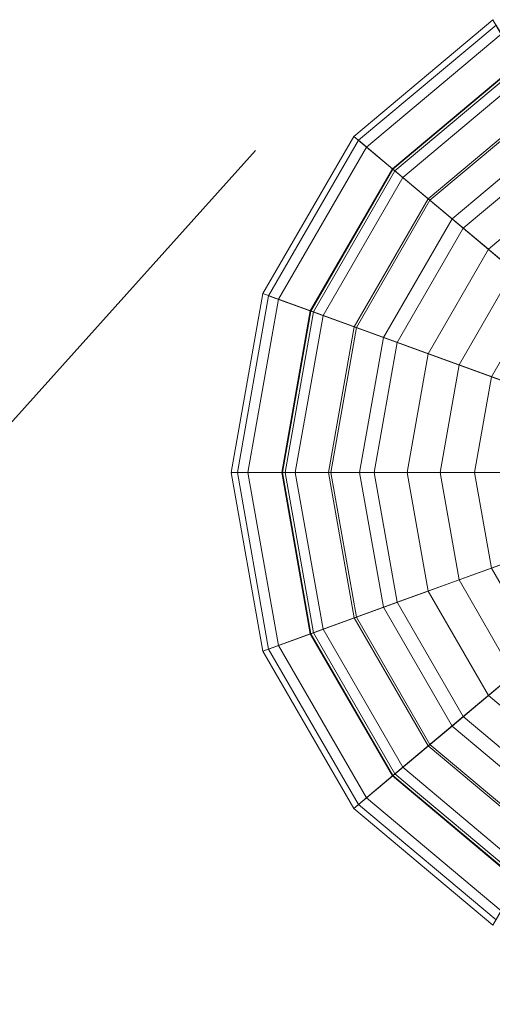
# Model space of a CAD drawing. Units: inches. Extents: x 375 to 1122, y 27 to 1069.
# Tile 57 of 155: x 731.16 to 732.383, y 305.711 to 308.262. Entities that reach past the tile are written whole.
import ezdxf

# ---------------------------------------------------------------- set-up
doc = ezdxf.new("R2010")
doc.units = ezdxf.units.IN
doc.layers.add('Furniture', color=30, linetype='Continuous', lineweight=18)

# ---------------------------------------------------------------- blocks, each defined once
blk = doc.blocks.new('A$C403C54AD')
blk.add_line((0.959313, 1.170619, -0.000599), (1.358468, 0.812559, -0.000599))
for points in [[(0.950832, 1.185986, -0.04658), (0.980157, 1.202917, -0.043501), (0.980157, 1.202917, -0.043501), (0.958391, 1.176977, -0.04658)], [(0.958391, 1.176977, -0.04658), (0.980157, 1.202917, -0.043501), (0.980157, 1.202917, -0.043501), (0.968576, 1.171097, -0.04658)], [(0.968576, 1.171097, -0.04658), (0.980157, 1.202917, -0.043501), (0.980157, 1.202917, -0.043501), (0.980157, 1.169055, -0.04658)], [(1.001923, 1.176977, -0.04658), (0.980157, 1.202917, -0.043501), (0.980157, 1.202917, -0.043501), (1.009483, 1.185986, -0.04658)], [(0.991739, 1.171097, -0.04658), (0.980157, 1.202917, -0.043501), (0.980157, 1.202917, -0.043501), (1.001923, 1.176977, -0.04658)], [(0.980157, 1.169055, -0.04658), (0.980157, 1.202917, -0.043501), (0.980157, 1.202917, -0.043501), (0.991739, 1.171097, -0.04658)], [(0.974434, 1.196096, 0.042248), (0.968505, 1.189031, 0.048884), (0.973957, 1.185883, 0.048884), (0.977112, 1.19455, 0.042248)], [(0.983203, 1.19455, 0.042248), (0.986357, 1.185883, 0.048884), (0.991809, 1.189031, 0.048884), (0.985881, 1.196096, 0.042248)], [(0.967847, 1.19581, -0.040074), (0.95366, 1.187619, -0.043349), (0.96049, 1.179479, -0.043349), (0.971021, 1.192029, -0.040074)], [(0.989294, 1.192029, -0.040074), (0.999824, 1.179479, -0.043349), (1.006655, 1.187619, -0.043349), (0.992467, 1.19581, -0.040074)], [(0.967072, 1.187323, 0.046697), (0.973653, 1.195166, 0.03933), (0.976696, 1.193409, 0.03933), (0.973195, 1.183788, 0.046697)], [(0.98712, 1.183788, 0.046697), (0.983618, 1.193409, 0.03933), (0.986661, 1.195166, 0.03933), (0.993243, 1.187323, 0.046697)], [(0.977112, 1.19455, 0.042248), (0.973957, 1.185883, 0.048884), (0.980157, 1.18479, 0.048884), (0.980157, 1.194013, 0.042248)], [(0.980157, 1.194013, 0.042248), (0.980157, 1.18479, 0.048884), (0.986357, 1.185883, 0.048884), (0.983203, 1.19455, 0.042248)], [(0.964459, 1.193854, 0.048884), (0.958842, 1.190611, 0.058276), (0.964336, 1.184063, 0.058276), (0.968505, 1.189031, 0.048884)], [(0.973195, 1.183788, 0.046697), (0.976696, 1.193409, 0.03933), (0.980157, 1.192799, 0.03933), (0.980157, 1.18256, 0.046697)], [(0.980157, 1.18256, 0.046697), (0.980157, 1.192799, 0.03933), (0.983618, 1.193409, 0.03933), (0.98712, 1.183788, 0.046697)], [(0.991809, 1.189031, 0.048884), (0.995978, 1.184063, 0.058276), (1.001473, 1.190611, 0.058276), (0.995856, 1.193854, 0.048884)], [(0.956408, 1.189206, 0.056929), (0.962527, 1.192739, 0.046697), (0.967072, 1.187323, 0.046697), (0.96253, 1.18191, 0.056929)], [(0.997785, 1.18191, 0.056929), (0.993243, 1.187323, 0.046697), (0.997787, 1.192739, 0.046697), (1.003907, 1.189206, 0.056929)], [(0.956282, 1.189133, 0.115599), (0.960688, 1.191677, 0.12581), (0.965707, 1.185696, 0.12581), (0.962436, 1.181798, 0.115599)], [(0.960688, 1.191677, 0.12581), (0.958022, 1.190138, 0.12581), (0.963728, 1.183338, 0.12581), (0.965707, 1.185696, 0.12581)], [(0.971021, 1.192029, -0.040074), (0.96049, 1.179479, -0.043349), (0.969693, 1.174166, -0.043349), (0.975296, 1.18956, -0.040074)], [(0.985019, 1.18956, -0.040074), (0.990622, 1.174166, -0.043349), (0.999824, 1.179479, -0.043349), (0.989294, 1.192029, -0.040074)], [(0.994608, 1.185696, 0.12581), (0.996587, 1.183338, 0.12581), (1.002293, 1.190138, 0.12581), (0.999627, 1.191677, 0.12581)], [(0.997878, 1.181798, 0.115599), (0.994608, 1.185696, 0.12581), (0.999627, 1.191677, 0.12581), (1.004033, 1.189133, 0.115599)], [(0.958842, 1.190611, 0.058276), (0.954418, 1.188057, 0.075423), (0.961053, 1.18015, 0.075423), (0.964336, 1.184063, 0.058276)], [(0.995978, 1.184063, 0.058276), (0.999261, 1.18015, 0.075423), (1.005896, 1.188057, 0.075423), (1.001473, 1.190611, 0.058276)], [(0.958022, 1.190138, 0.12581), (0.953695, 1.187639, 0.116404), (0.960516, 1.17951, 0.116404), (0.963728, 1.183338, 0.12581)], [(0.975296, 1.18956, -0.040074), (0.969693, 1.174166, -0.043349), (0.980157, 1.172321, -0.043349), (0.980157, 1.188703, -0.040074)], [(0.980157, 1.188703, -0.040074), (0.980157, 1.172321, -0.043349), (0.990622, 1.174166, -0.043349), (0.985019, 1.18956, -0.040074)], [(0.996587, 1.183338, 0.12581), (0.999798, 1.17951, 0.116404), (1.00662, 1.187639, 0.116404), (1.002293, 1.190138, 0.12581)], [(0.951762, 1.186523, 0.074938), (0.956408, 1.189206, 0.056929), (0.96253, 1.18191, 0.056929), (0.959081, 1.1778, 0.074938)], [(0.953848, 1.187728, 0.102963), (0.956282, 1.189133, 0.115599), (0.962436, 1.181798, 0.115599), (0.96063, 1.179646, 0.102963)], [(0.968505, 1.189031, 0.048884), (0.964336, 1.184063, 0.058276), (0.971739, 1.179789, 0.058276), (0.973957, 1.185883, 0.048884)], [(0.986357, 1.185883, 0.048884), (0.988575, 1.179789, 0.058276), (0.995978, 1.184063, 0.058276), (0.991809, 1.189031, 0.048884)], [(1.001233, 1.1778, 0.074938), (0.997785, 1.18191, 0.056929), (1.003907, 1.189206, 0.056929), (1.008553, 1.186523, 0.074938)], [(0.999684, 1.179646, 0.102963), (0.997878, 1.181798, 0.115599), (1.004033, 1.189133, 0.115599), (1.006466, 1.187728, 0.102963)], [(0.953695, 1.187639, 0.116404), (0.951177, 1.186186, 0.10318), (0.958647, 1.177283, 0.10318), (0.960516, 1.17951, 0.116404)], [(0.954418, 1.188057, 0.075423), (0.953848, 1.187728, 0.102963), (0.96063, 1.179646, 0.102963), (0.961053, 1.18015, 0.075423)], [(0.999261, 1.18015, 0.075423), (0.999684, 1.179646, 0.102963), (1.006466, 1.187728, 0.102963), (1.005896, 1.188057, 0.075423)], [(0.999798, 1.17951, 0.116404), (1.001667, 1.177283, 0.10318), (1.009137, 1.186186, 0.10318), (1.00662, 1.187639, 0.116404)], [(0.95366, 1.187619, -0.043349), (0.950832, 1.185986, -0.04658), (0.958391, 1.176977, -0.04658), (0.96049, 1.179479, -0.043349)], [(0.96253, 1.18191, 0.056929), (0.967072, 1.187323, 0.046697), (0.973195, 1.183788, 0.046697), (0.970778, 1.177147, 0.056929)], [(0.989537, 1.177147, 0.056929), (0.98712, 1.183788, 0.046697), (0.993243, 1.187323, 0.046697), (0.997785, 1.18191, 0.056929)], [(0.999824, 1.179479, -0.043349), (1.001923, 1.176977, -0.04658), (1.009483, 1.185986, -0.04658), (1.006655, 1.187619, -0.043349)], [(0.951177, 1.186186, 0.10318), (0.951762, 1.186523, 0.074938), (0.959081, 1.1778, 0.074938), (0.958647, 1.177283, 0.10318)], [(1.001667, 1.177283, 0.10318), (1.001233, 1.1778, 0.074938), (1.008553, 1.186523, 0.074938), (1.009137, 1.186186, 0.10318)], [(0.973957, 1.185883, 0.048884), (0.971739, 1.179789, 0.058276), (0.980157, 1.178304, 0.058276), (0.980157, 1.18479, 0.048884)], [(0.980157, 1.18479, 0.048884), (0.980157, 1.178304, 0.058276), (0.988575, 1.179789, 0.058276), (0.986357, 1.185883, 0.048884)], [(0.962436, 1.181798, 0.115599), (0.965707, 1.185696, 0.12581), (0.972468, 1.181792, 0.12581), (0.970728, 1.177011, 0.115599)], [(0.965707, 1.185696, 0.12581), (0.963728, 1.183338, 0.12581), (0.971415, 1.178899, 0.12581), (0.972468, 1.181792, 0.12581)], [(0.987846, 1.181792, 0.12581), (0.988899, 1.178899, 0.12581), (0.996587, 1.183338, 0.12581), (0.994608, 1.185696, 0.12581)], [(0.989586, 1.177011, 0.115599), (0.987846, 1.181792, 0.12581), (0.994608, 1.185696, 0.12581), (0.997878, 1.181798, 0.115599)], [(0.964336, 1.184063, 0.058276), (0.961053, 1.18015, 0.075423), (0.969992, 1.174989, 0.075423), (0.971739, 1.179789, 0.058276)], [(0.988575, 1.179789, 0.058276), (0.990322, 1.174989, 0.075423), (0.999261, 1.18015, 0.075423), (0.995978, 1.184063, 0.058276)], [(0.963728, 1.183338, 0.12581), (0.960516, 1.17951, 0.116404), (0.969706, 1.174204, 0.116404), (0.971415, 1.178899, 0.12581)], [(0.970778, 1.177147, 0.056929), (0.973195, 1.183788, 0.046697), (0.980157, 1.18256, 0.046697), (0.980157, 1.175494, 0.056929)], [(0.980157, 1.175494, 0.056929), (0.980157, 1.18256, 0.046697), (0.98712, 1.183788, 0.046697), (0.989537, 1.177147, 0.056929)], [(0.988899, 1.178899, 0.12581), (0.990608, 1.174204, 0.116404), (0.999798, 1.17951, 0.116404), (0.996587, 1.183338, 0.12581)], [(0.959081, 1.1778, 0.074938), (0.96253, 1.18191, 0.056929), (0.970778, 1.177147, 0.056929), (0.968943, 1.172106, 0.074938)], [(0.991372, 1.172106, 0.074938), (0.989537, 1.177147, 0.056929), (0.997785, 1.18191, 0.056929), (1.001233, 1.1778, 0.074938)], [(0.96063, 1.179646, 0.102963), (0.962436, 1.181798, 0.115599), (0.970728, 1.177011, 0.115599), (0.969767, 1.174371, 0.102963)], [(0.970728, 1.177011, 0.115599), (0.972468, 1.181792, 0.12581), (0.980157, 1.180436, 0.12581), (0.980157, 1.175348, 0.115599)], [(0.972468, 1.181792, 0.12581), (0.971415, 1.178899, 0.12581), (0.980157, 1.177358, 0.12581), (0.980157, 1.180436, 0.12581)], [(0.980157, 1.180436, 0.12581), (0.980157, 1.177358, 0.12581), (0.988899, 1.178899, 0.12581), (0.987846, 1.181792, 0.12581)], [(0.980157, 1.175348, 0.115599), (0.980157, 1.180436, 0.12581), (0.987846, 1.181792, 0.12581), (0.989586, 1.177011, 0.115599)], [(0.990547, 1.174371, 0.102963), (0.989586, 1.177011, 0.115599), (0.997878, 1.181798, 0.115599), (0.999684, 1.179646, 0.102963)], [(0.961053, 1.18015, 0.075423), (0.96063, 1.179646, 0.102963), (0.969767, 1.174371, 0.102963), (0.969992, 1.174989, 0.075423)], [(0.990322, 1.174989, 0.075423), (0.990547, 1.174371, 0.102963), (0.999684, 1.179646, 0.102963), (0.999261, 1.18015, 0.075423)], [(0.96049, 1.179479, -0.043349), (0.958391, 1.176977, -0.04658), (0.968576, 1.171097, -0.04658), (0.969693, 1.174166, -0.043349)], [(0.960516, 1.17951, 0.116404), (0.958647, 1.177283, 0.10318), (0.968712, 1.171472, 0.10318), (0.969706, 1.174204, 0.116404)], [(0.971739, 1.179789, 0.058276), (0.969992, 1.174989, 0.075423), (0.980157, 1.173197, 0.075423), (0.980157, 1.178304, 0.058276)], [(0.980157, 1.178304, 0.058276), (0.980157, 1.173197, 0.075423), (0.990322, 1.174989, 0.075423), (0.988575, 1.179789, 0.058276)], [(0.990608, 1.174204, 0.116404), (0.991602, 1.171472, 0.10318), (1.001667, 1.177283, 0.10318), (0.999798, 1.17951, 0.116404)], [(0.990622, 1.174166, -0.043349), (0.991739, 1.171097, -0.04658), (1.001923, 1.176977, -0.04658), (0.999824, 1.179479, -0.043349)], [(0.971415, 1.178899, 0.12581), (0.969706, 1.174204, 0.116404), (0.980157, 1.172361, 0.116404), (0.980157, 1.177358, 0.12581)], [(0.980157, 1.177358, 0.12581), (0.980157, 1.172361, 0.116404), (0.990608, 1.174204, 0.116404), (0.988899, 1.178899, 0.12581)], [(0.958647, 1.177283, 0.10318), (0.959081, 1.1778, 0.074938), (0.968943, 1.172106, 0.074938), (0.968712, 1.171472, 0.10318)], [(0.991602, 1.171472, 0.10318), (0.991372, 1.172106, 0.074938), (1.001233, 1.1778, 0.074938), (1.001667, 1.177283, 0.10318)], [(0.968943, 1.172106, 0.074938), (0.970778, 1.177147, 0.056929), (0.980157, 1.175494, 0.056929), (0.980157, 1.170129, 0.074938)], [(0.969767, 1.174371, 0.102963), (0.970728, 1.177011, 0.115599), (0.980157, 1.175348, 0.115599), (0.980157, 1.172539, 0.102963)], [(0.980157, 1.170129, 0.074938), (0.980157, 1.175494, 0.056929), (0.989537, 1.177147, 0.056929), (0.991372, 1.172106, 0.074938)], [(0.980157, 1.172539, 0.102963), (0.980157, 1.175348, 0.115599), (0.989586, 1.177011, 0.115599), (0.990547, 1.174371, 0.102963)], [(0.969992, 1.174989, 0.075423), (0.969767, 1.174371, 0.102963), (0.980157, 1.172539, 0.102963), (0.980157, 1.173197, 0.075423)], [(0.980157, 1.173197, 0.075423), (0.980157, 1.172539, 0.102963), (0.990547, 1.174371, 0.102963), (0.990322, 1.174989, 0.075423)], [(0.969693, 1.174166, -0.043349), (0.968576, 1.171097, -0.04658), (0.980157, 1.169055, -0.04658), (0.980157, 1.172321, -0.043349)], [(0.969706, 1.174204, 0.116404), (0.968712, 1.171472, 0.10318), (0.980157, 1.169454, 0.10318), (0.980157, 1.172361, 0.116404)], [(0.980157, 1.172361, 0.116404), (0.980157, 1.169454, 0.10318), (0.991602, 1.171472, 0.10318), (0.990608, 1.174204, 0.116404)], [(0.980157, 1.172321, -0.043349), (0.980157, 1.169055, -0.04658), (0.991739, 1.171097, -0.04658), (0.990622, 1.174166, -0.043349)], [(0.968712, 1.171472, 0.10318), (0.968943, 1.172106, 0.074938), (0.980157, 1.170129, 0.074938), (0.980157, 1.169454, 0.10318)], [(0.980157, 1.169454, 0.10318), (0.980157, 1.170129, 0.074938), (0.991372, 1.172106, 0.074938), (0.991602, 1.171472, 0.10318)]]:
    blk.add_3dface(points)

msp = doc.modelspace()

# ---------------------------------------------------------------- block references
at = {"layer": 'Furniture', "xscale": 39.9918517141215, "yscale": 39.9918517141215, "zscale": 39.9918517141215, "rotation": 270}
msp.add_blockref('A$C403C54AD', (684.9549, 346.2875, 0.024), dxfattribs=at)

doc.saveas('drawing.dxf')
